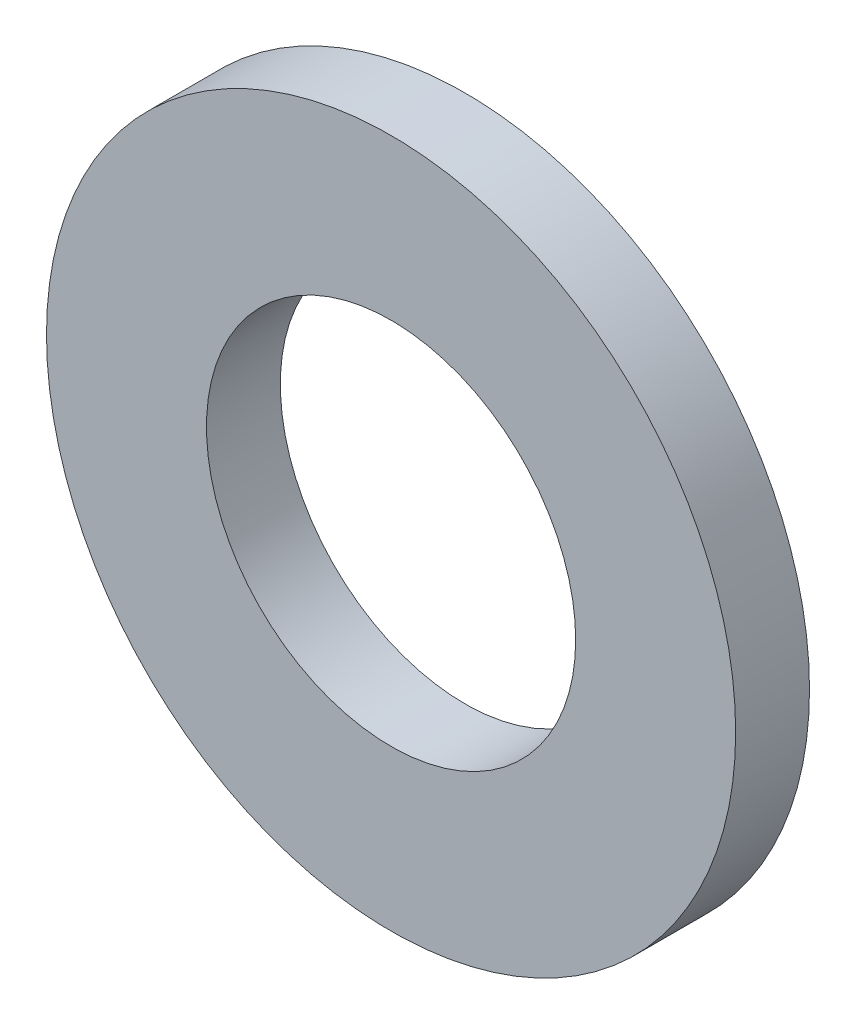
SolidWorks part; units mm, degrees
material "Plain Carbon Steel"
ref_plane "Front Plane" through (0, 0, 0) normal (0, 0, 1) x (1, 0, 0)
ref_plane "Top Plane" through (0, 0, 0) normal (0, 1, 0) x (1, 0, 0)
ref_plane "Right Plane" through (0, 0, 0) normal (1, 0, 0) x (0, 0, -1)
sketch "Washer Profile Ø28-Ø15" plane through (0, 0, 0) normal (0, 0, 1) x (1, 0, 0)
  circle A0 centre (0, 0) radius 14
  circle A1 centre (0, 0) radius 7.5
  dimension "D1" = 28
  dimension "D2" = 15
extrude "Washer Body 3mm" add sketch "Washer Profile Ø28-Ø15" along normal mid plane 3
